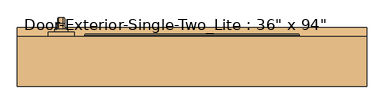
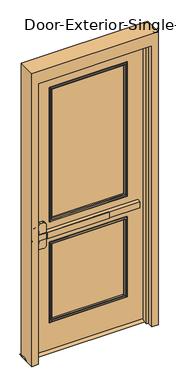
"""IFC4 building model written with IfcOpenShell, lengths in millimetres: door geometry."""

from ifc_helpers import new_model, si_unit, point, frame, frame_2d, origin, place, context, project, spatial, polyline, circle_curve, ellipse_curve, trimmed, segment, composite_curve, outline, extrude, faceted_brep, source, transform, mapped, element, save
from ifc_brep_helpers import plane_surface, cylinder_surface, revolved_surface, advanced_brep


def door_b6c2ee01(model_context):
    return source(origin(), model_context, "Body", "SolidModel", [
        extrude(outline(polyline([(38.1, 12.7), (82.55, 12.7), (107.95, 0.0), (12.7, 0.0), (38.1, 12.7)])), frame((-508.0, 0.0, 0.0), z_axis=(1.0, 0.0, 0.0), x_axis=(0.0, 1.0, 0.0)), (0.0, 0.0, 1.0), 1016.0),
        extrude(outline(polyline([(150.2833333, 0.0), (-349.25, 0.0), (-349.25, 6.35), (150.2833333, 6.35), (150.2833333, 0.0)])), frame((0.0, 0.0, 990.6), z_axis=(0.0, 0.0, 1.0), x_axis=(1.0, 0.0, 0.0)), (0.0, 0.0, 1.0), 50.8),
        advanced_brep(
        [(-412.75, 6.35, 1041.4), (-412.75, 6.35, 990.6), (-349.25, 6.35, 990.6), (400.05, 6.35, 990.6), (400.05, 6.35, 1041.4), (-349.25, 6.35, 1041.4), (400.05, 38.1, 1041.4), (400.05, 38.1, 990.6), (-349.25, 38.1, 990.6), (-349.25, 38.1, 927.1), (-368.3, 38.1, 908.05), (-393.7, 38.1, 908.05), (-412.75, 38.1, 927.1), (-412.75, 38.1, 1104.9), (-393.7, 38.1, 1123.95), (-368.3, 38.1, 1123.95), (-349.25, 38.1, 1104.9), (-349.25, 38.1, 1041.4), (-349.25, 9.5252467, 1041.4), (-412.75, 9.5252467, 1041.4), (-412.75, 14.5354269, 1104.9), (-412.75, 14.5354269, 927.1), (-412.75, 9.5252467, 990.6), (-349.25, 9.5252467, 990.6), (-349.25, 14.5354269, 927.1), (-349.25, 14.5354269, 1104.9), (-393.7, 16.038481, 1123.95), (-368.3, 16.038481, 1123.95), (-368.3, 16.038481, 908.05), (-393.7, 16.038481, 908.05)],
        [
            (0, 1),
            (1, 2),
            (2, 3),
            (3, 4),
            (4, 5),
            (5, 0),
            (6, 7),
            (7, 8),
            (8, 9),
            (9, 10, circle_curve(frame((-368.3, 38.1, 927.1), z_axis=(0.0, 1.0, 0.0), x_axis=(1.0, 0.0, 0.0)), 19.05)),
            (10, 11),
            (11, 12, circle_curve(frame((-393.7, 38.1, 927.1), z_axis=(0.0, 1.0, 0.0), x_axis=(1.0, 0.0, 0.0)), 19.05)),
            (12, 13),
            (13, 14, circle_curve(frame((-393.7, 38.1, 1104.9), z_axis=(0.0, 1.0, 0.0), x_axis=(1.0, 0.0, 0.0)), 19.05)),
            (14, 15),
            (15, 16, circle_curve(frame((-368.3, 38.1, 1104.9), z_axis=(0.0, 1.0, 0.0), x_axis=(1.0, 0.0, 0.0)), 19.05)),
            (16, 17),
            (17, 6),
            (4, 6),
            (17, 18),
            (18, 19),
            (19, 0),
            (19, 20),
            (20, 13),
            (12, 21),
            (21, 22),
            (22, 1),
            (7, 3),
            (22, 23),
            (23, 8),
            (23, 24),
            (24, 9),
            (16, 25),
            (25, 18),
            (14, 26),
            (26, 27),
            (27, 15),
            (10, 28),
            (28, 29),
            (29, 11),
            (24, 28, ellipse_curve(frame((-368.3, 14.5354269, 927.1), z_axis=(0.0, 0.9969018152893365, 0.07865602756830282), x_axis=(0.0, -0.07865602756830208, 0.9969018152893365)), 19.1092038, 19.05)),
            (27, 25, ellipse_curve(frame((-368.3, 14.5354269, 1104.9), z_axis=(0.0, 0.9969018152893376, -0.07865602756828934), x_axis=(0.0, -0.078656027568288, -0.9969018152893377)), 19.1092038, 19.05)),
            (20, 26, ellipse_curve(frame((-393.7, 14.5354269, 1104.9), z_axis=(0.0, 0.9969018152893376, -0.07865602756828934), x_axis=(0.0, -0.078656027568288, -0.9969018152893377)), 19.1092038, 19.05)),
            (29, 21, ellipse_curve(frame((-393.7, 14.5354269, 927.1), z_axis=(0.0, 0.9969018152893365, 0.07865602756830282), x_axis=(0.0, -0.07865602756830208, 0.9969018152893365)), 19.1092038, 19.05)),
        ],
        [
            plane_surface(frame((-412.75, 6.35, 1041.4), z_axis=(0.0, -1.0, 0.0), x_axis=(-1.0, 0.0, 0.0))),
            plane_surface(frame((-412.75, 38.1, 1041.4), z_axis=(0.0, 1.0, 0.0), x_axis=(1.0, 0.0, 0.0))),
            plane_surface(frame((400.05, 6.35, 1041.4), z_axis=(0.0, 0.0, 1.0), x_axis=(0.0, 1.0, 0.0))),
            plane_surface(frame((-412.75, 6.35, 1041.4), z_axis=(-1.0, 0.0, 0.0), x_axis=(0.0, 1.0, 0.0))),
            plane_surface(frame((-412.75, 6.35, 990.6), z_axis=(0.0, 0.0, -1.0), x_axis=(0.0, 1.0, 0.0))),
            plane_surface(frame((400.05, 6.35, 990.6), z_axis=(1.0, 0.0, 0.0), x_axis=(0.0, 1.0, 0.0))),
            plane_surface(frame((-349.25, 9.5252467, 927.1), z_axis=(1.0, 0.0, 0.0), x_axis=(0.0, 1.0, 0.0))),
            plane_surface(frame((-368.3, 9.5252467, 1123.95), z_axis=(0.0, 0.0, 1.0), x_axis=(0.0, 1.0, 0.0))),
            plane_surface(frame((-393.7, 9.5252467, 908.05), z_axis=(0.0, 0.0, -1.0), x_axis=(0.0, 1.0, 0.0))),
            cylinder_surface(frame((-368.3, 38.1, 927.1), z_axis=(0.0, -1.0, 0.0), x_axis=(1.0, 0.0, 0.0)), 19.05),
            cylinder_surface(frame((-368.3, 38.1, 1104.9), z_axis=(0.0, -1.0, 0.0), x_axis=(1.0, 0.0, 0.0)), 19.05),
            cylinder_surface(frame((-393.7, 38.1, 1104.9), z_axis=(0.0, -1.0, 0.0), x_axis=(1.0, 0.0, 0.0)), 19.05),
            cylinder_surface(frame((-393.7, 38.1, 927.1), z_axis=(0.0, -1.0, 0.0), x_axis=(1.0, 0.0, 0.0)), 19.05),
            plane_surface(frame((-349.25, 9.5252467, 1041.4), z_axis=(0.0, -0.9969018152893376, 0.07865602756828934), x_axis=(-1.0, 0.0, 0.0))),
            plane_surface(frame((-349.25, 16.038481, 908.05), z_axis=(0.0, -0.9969018152893365, -0.07865602756830282), x_axis=(-1.0, 0.0, 0.0))),
        ],
        [
            (0, [[1, 2, 3, 4, 5, 6]]),
            (1, [[7, 8, 9, 10, 11, 12, 13, 14, 15, 16, 17, 18]]),
            (2, [[19, -18, 20, 21, 22, -6, -5]]),
            (3, [[-1, -22, 23, 24, -13, 25, 26, 27]]),
            (4, [[28, -3, -2, -27, 29, 30, -8]]),
            (5, [[-4, -28, -7, -19]]),
            (6, [[-9, -30, 31, 32]]),
            (6, [[-17, 33, 34, -20]]),
            (7, [[-15, 35, 36, 37]]),
            (8, [[-11, 38, 39, 40]]),
            (9, [[-10, -32, 41, -38]]),
            (10, [[-16, -37, 42, -33]]),
            (11, [[-14, -24, 43, -35]]),
            (12, [[-12, -40, 44, -25]]),
            (13, [[-21, -34, -42, -36, -43, -23]]),
            (14, [[-26, -44, -39, -41, -31, -29]]),
        ],
    ),
        advanced_brep(
        [(-391.0, 95.25, 1017.190625), (-391.0, 95.25, 1014.809375), (-387.428125, 95.25, 1011.2375), (-374.5715406, 95.25, 1011.2375), (-371.0, 95.25, 1014.8090406), (-371.0, 95.25, 1017.190625), (-374.571875, 95.25, 1020.7625), (-387.428125, 95.25, 1020.7625), (-391.0, 95.25, 887.809375), (-387.428125, 95.25, 884.2375), (-374.571875, 95.25, 884.2375), (-371.0, 95.25, 887.809375), (-371.0, 95.25, 890.1909594), (-374.5715406, 95.25, 893.7625), (-387.428125, 95.25, 893.7625), (-391.0, 95.25, 890.190625), (-391.0, 120.65, 1017.190625), (-391.0, 134.540625, 1003.3), (-391.0, 134.540625, 901.7), (-391.0, 120.65, 887.809375), (-391.0, 120.65, 890.190625), (-391.0, 132.159375, 901.7), (-391.0, 132.159375, 1003.3), (-391.0, 120.65, 1014.809375), (-387.428125, 120.65, 1011.2375), (-374.5715406, 120.65, 1011.2375), (-371.0, 120.65, 1014.8090406), (-371.0, 132.1590406, 1003.3), (-371.0, 132.1590406, 901.7), (-371.0, 120.65, 890.1909594), (-371.0, 120.65, 887.809375), (-371.0, 134.540625, 901.7), (-371.0, 134.540625, 1003.3), (-371.0, 120.65, 1017.190625), (-374.571875, 120.65, 1020.7625), (-387.428125, 120.65, 1020.7625), (-387.428125, 128.5875, 1003.3), (-374.5715406, 128.5875, 1003.3), (-374.571875, 138.1125, 1003.3), (-387.428125, 138.1125, 1003.3), (-387.428125, 128.5875, 901.7), (-374.5715406, 128.5875, 901.7), (-374.571875, 138.1125, 901.7), (-387.428125, 138.1125, 901.7), (-387.428125, 120.65, 893.7625), (-374.5715406, 120.65, 893.7625), (-374.571875, 120.65, 884.2375), (-387.428125, 120.65, 884.2375)],
        [
            (0, 1),
            (1, 2, circle_curve(frame((-387.428125, 95.25, 1014.809375), z_axis=(0.0, -1.0, 0.0), x_axis=(0.0, 0.0, 1.0)), 3.571875)),
            (2, 3),
            (3, 4, circle_curve(frame((-374.5715406, 95.25, 1014.8090406), z_axis=(0.0, -1.0, 0.0), x_axis=(0.0, 0.0, 1.0)), 3.5715406)),
            (4, 5),
            (5, 6, circle_curve(frame((-374.571875, 95.25, 1017.190625), z_axis=(0.0, -1.0, 0.0), x_axis=(0.0, 0.0, 1.0)), 3.571875)),
            (6, 7),
            (7, 0, circle_curve(frame((-387.428125, 95.25, 1017.190625), z_axis=(0.0, -1.0, 0.0), x_axis=(0.0, 0.0, 1.0)), 3.571875)),
            (8, 9, circle_curve(frame((-387.428125, 95.25, 887.809375), z_axis=(0.0, -1.0, 0.0), x_axis=(0.0, 0.0, -1.0)), 3.571875)),
            (9, 10),
            (10, 11, circle_curve(frame((-374.571875, 95.25, 887.809375), z_axis=(0.0, -1.0, 0.0), x_axis=(0.0, 0.0, -1.0)), 3.571875)),
            (11, 12),
            (12, 13, circle_curve(frame((-374.5715406, 95.25, 890.1909594), z_axis=(0.0, -1.0, 0.0), x_axis=(0.0, 0.0, -1.0)), 3.5715406)),
            (13, 14),
            (14, 15, circle_curve(frame((-387.428125, 95.25, 890.190625), z_axis=(0.0, -1.0, 0.0), x_axis=(0.0, 0.0, -1.0)), 3.571875)),
            (15, 8),
            (0, 16),
            (16, 17, circle_curve(frame((-391.0, 120.65, 1003.3), z_axis=(-1.0, 0.0, 0.0), x_axis=(0.0, 0.0, 1.0)), 13.890625)),
            (17, 18),
            (18, 19, circle_curve(frame((-391.0, 120.65, 901.7), z_axis=(-1.0, 0.0, 0.0), x_axis=(0.0, 1.0, 0.0)), 13.890625)),
            (19, 8),
            (15, 20),
            (20, 21, circle_curve(frame((-391.0, 120.65, 901.7), z_axis=(1.0, 0.0, 0.0), x_axis=(0.0, 1.0, 0.0)), 11.509375)),
            (21, 22),
            (22, 23, circle_curve(frame((-391.0, 120.65, 1003.3), z_axis=(1.0, 0.0, 0.0), x_axis=(0.0, 0.0, 1.0)), 11.509375)),
            (23, 1),
            (23, 24, circle_curve(frame((-387.428125, 120.65, 1014.809375), z_axis=(0.0, -1.0, 0.0), x_axis=(0.0, 0.0, 1.0)), 3.571875)),
            (24, 2),
            (24, 25),
            (25, 3),
            (25, 26, circle_curve(frame((-374.5715406, 120.65, 1014.8090406), z_axis=(0.0, -1.0, 0.0), x_axis=(0.0, 0.0, 1.0)), 3.5715406)),
            (26, 4),
            (26, 27, circle_curve(frame((-371.0, 120.65, 1003.3), z_axis=(-1.0, 0.0, 0.0), x_axis=(0.0, 0.0, 1.0)), 11.5090406)),
            (27, 28),
            (28, 29, circle_curve(frame((-371.0, 120.65, 901.7), z_axis=(-1.0, 0.0, 0.0), x_axis=(0.0, 1.0, 0.0)), 11.5090406)),
            (29, 12),
            (11, 30),
            (30, 31, circle_curve(frame((-371.0, 120.65, 901.7), z_axis=(1.0, 0.0, 0.0), x_axis=(0.0, 1.0, 0.0)), 13.890625)),
            (31, 32),
            (32, 33, circle_curve(frame((-371.0, 120.65, 1003.3), z_axis=(1.0, 0.0, 0.0), x_axis=(0.0, 0.0, 1.0)), 13.890625)),
            (33, 5),
            (33, 34, circle_curve(frame((-374.571875, 120.65, 1017.190625), z_axis=(0.0, -1.0, 0.0), x_axis=(0.0, 0.0, 1.0)), 3.571875)),
            (34, 6),
            (34, 35),
            (35, 7),
            (35, 16, circle_curve(frame((-387.428125, 120.65, 1017.190625), z_axis=(0.0, -1.0, 0.0), x_axis=(0.0, 0.0, 1.0)), 3.571875)),
            (36, 24, circle_curve(frame((-387.428125, 120.65, 1003.3), z_axis=(1.0, 0.0, 0.0), x_axis=(0.0, 0.0, 1.0)), 7.9375)),
            (22, 36, circle_curve(frame((-387.428125, 132.159375, 1003.3), z_axis=(0.0, 0.0, 1.0), x_axis=(0.0, 1.0, 0.0)), 3.571875)),
            (37, 25, circle_curve(frame((-374.5715406, 120.65, 1003.3), z_axis=(1.0, 0.0, 0.0), x_axis=(0.0, 0.0, 1.0)), 7.9375)),
            (36, 37),
            (37, 27, circle_curve(frame((-374.5715406, 132.1590406, 1003.3), z_axis=(0.0, 0.0, 1.0), x_axis=(0.0, 1.0, 0.0)), 3.5715406)),
            (38, 34, circle_curve(frame((-374.571875, 120.65, 1003.3), z_axis=(1.0, 0.0, 0.0), x_axis=(0.0, 0.0, 1.0)), 17.4625)),
            (32, 38, circle_curve(frame((-374.571875, 134.540625, 1003.3), z_axis=(0.0, 0.0, 1.0), x_axis=(0.0, 1.0, 0.0)), 3.571875)),
            (39, 35, circle_curve(frame((-387.428125, 120.65, 1003.3), z_axis=(1.0, 0.0, 0.0), x_axis=(0.0, 0.0, 1.0)), 17.4625)),
            (38, 39),
            (39, 17, circle_curve(frame((-387.428125, 134.540625, 1003.3), z_axis=(0.0, 0.0, 1.0), x_axis=(0.0, 1.0, 0.0)), 3.571875)),
            (21, 40, circle_curve(frame((-387.428125, 132.159375, 901.7), z_axis=(0.0, 0.0, 1.0), x_axis=(0.0, 1.0, 0.0)), 3.571875)),
            (40, 36),
            (40, 41),
            (41, 37),
            (41, 28, circle_curve(frame((-374.5715406, 132.1590406, 901.7), z_axis=(0.0, 0.0, 1.0), x_axis=(0.0, 1.0, 0.0)), 3.5715406)),
            (31, 42, circle_curve(frame((-374.571875, 134.540625, 901.7), z_axis=(0.0, 0.0, 1.0), x_axis=(0.0, 1.0, 0.0)), 3.571875)),
            (42, 38),
            (42, 43),
            (43, 39),
            (43, 18, circle_curve(frame((-387.428125, 134.540625, 901.7), z_axis=(0.0, 0.0, 1.0), x_axis=(0.0, 1.0, 0.0)), 3.571875)),
            (44, 40, circle_curve(frame((-387.428125, 120.65, 901.7), z_axis=(1.0, 0.0, 0.0), x_axis=(0.0, 1.0, 0.0)), 7.9375)),
            (20, 44, circle_curve(frame((-387.428125, 120.65, 890.190625), z_axis=(0.0, 1.0, 0.0), x_axis=(0.0, 0.0, -1.0)), 3.571875)),
            (45, 41, circle_curve(frame((-374.5715406, 120.65, 901.7), z_axis=(1.0, 0.0, 0.0), x_axis=(0.0, 1.0, 0.0)), 7.9375)),
            (44, 45),
            (45, 29, circle_curve(frame((-374.5715406, 120.65, 890.1909594), z_axis=(0.0, 1.0, 0.0), x_axis=(0.0, 0.0, -1.0)), 3.5715406)),
            (46, 42, circle_curve(frame((-374.571875, 120.65, 901.7), z_axis=(1.0, 0.0, 0.0), x_axis=(0.0, 1.0, 0.0)), 17.4625)),
            (30, 46, circle_curve(frame((-374.571875, 120.65, 887.809375), z_axis=(0.0, 1.0, 0.0), x_axis=(0.0, 0.0, -1.0)), 3.571875)),
            (47, 43, circle_curve(frame((-387.428125, 120.65, 901.7), z_axis=(1.0, 0.0, 0.0), x_axis=(0.0, 1.0, 0.0)), 17.4625)),
            (46, 47),
            (47, 19, circle_curve(frame((-387.428125, 120.65, 887.809375), z_axis=(0.0, 1.0, 0.0), x_axis=(0.0, 0.0, -1.0)), 3.571875)),
            (14, 44),
            (13, 45),
            (10, 46),
            (9, 47),
        ],
        [
            plane_surface(frame((-381.0, 95.25, 1016.0), z_axis=(0.0, -1.0, 0.0), x_axis=(1.0, 0.0, 0.0))),
            plane_surface(frame((-381.0, 95.25, 889.0), z_axis=(0.0, -1.0, 0.0), x_axis=(1.0, 0.0, 0.0))),
            plane_surface(frame((-391.0, 95.25, 1017.190625), z_axis=(-1.0, 0.0, 0.0), x_axis=(0.0, 1.0, 0.0))),
            cylinder_surface(frame((-387.428125, 95.25, 1014.809375), z_axis=(0.0, -1.0, 0.0), x_axis=(0.0, 0.0, 1.0)), 3.571875),
            plane_surface(frame((-387.428125, 95.25, 1011.2375), z_axis=(0.0, 0.0, -1.0), x_axis=(0.0, 1.0, 0.0))),
            cylinder_surface(frame((-374.5715406, 95.25, 1014.8090406), z_axis=(0.0, -1.0, 0.0), x_axis=(0.0, 0.0, 1.0)), 3.5715406),
            plane_surface(frame((-371.0, 95.25, 1014.8090406), z_axis=(1.0, 0.0, 0.0), x_axis=(0.0, 1.0, 0.0))),
            cylinder_surface(frame((-374.571875, 95.25, 1017.190625), z_axis=(0.0, -1.0, 0.0), x_axis=(0.0, 0.0, 1.0)), 3.571875),
            plane_surface(frame((-374.571875, 95.25, 1020.7625), z_axis=(0.0, 0.0, 1.0), x_axis=(0.0, 1.0, 0.0))),
            cylinder_surface(frame((-387.428125, 95.25, 1017.190625), z_axis=(0.0, -1.0, 0.0), x_axis=(0.0, 0.0, 1.0)), 3.571875),
            revolved_surface(trimmed(ellipse_curve(frame((-387.428125, 120.65, 1014.809375), z_axis=(0.0, -1.0, 0.0), x_axis=(0.0, 0.0, 1.0)), 3.571875, 3.571875), [point((-391.0, 120.65, 1014.809375))], [point((-387.428125, 120.65, 1011.2375))], True, "CARTESIAN"), (-381.0, 120.65, 1003.3), (-1.0, 0.0, 0.0)),
            revolved_surface(polyline([(-387.428125, 120.65, 1011.2375), (-374.5715406, 120.65, 1011.2375)]), (-381.0, 120.65, 1003.3), (-1.0, 0.0, 0.0)),
            revolved_surface(trimmed(ellipse_curve(frame((-374.5715406, 120.65, 1014.8090406), z_axis=(0.0, -1.0, 0.0), x_axis=(0.0, 0.0, 1.0)), 3.5715406, 3.5715406), [point((-374.5715406, 120.65, 1011.2375))], [point((-371.0, 120.65, 1014.8090406))], True, "CARTESIAN"), (-381.0, 120.65, 1003.3), (-1.0, 0.0, 0.0)),
            revolved_surface(trimmed(ellipse_curve(frame((-374.571875, 120.65, 1017.190625), z_axis=(0.0, -1.0, 0.0), x_axis=(0.0, 0.0, 1.0)), 3.571875, 3.571875), [point((-371.0, 120.65, 1017.190625))], [point((-374.571875, 120.65, 1020.7625))], True, "CARTESIAN"), (-381.0, 120.65, 1003.3), (-1.0, 0.0, 0.0)),
            cylinder_surface(frame((-381.0, 120.65, 1003.3), z_axis=(-1.0, 0.0, 0.0), x_axis=(0.0, 0.0, 1.0)), 17.4625),
            revolved_surface(trimmed(ellipse_curve(frame((-387.428125, 120.65, 1017.190625), z_axis=(0.0, -1.0, 0.0), x_axis=(0.0, 0.0, 1.0)), 3.571875, 3.571875), [point((-387.428125, 120.65, 1020.7625))], [point((-391.0, 120.65, 1017.190625))], True, "CARTESIAN"), (-381.0, 120.65, 1003.3), (-1.0, 0.0, 0.0)),
            cylinder_surface(frame((-387.428125, 132.159375, 1003.3), z_axis=(0.0, 0.0, 1.0), x_axis=(0.0, 1.0, 0.0)), 3.571875),
            plane_surface(frame((-387.428125, 128.5875, 1003.3), z_axis=(0.0, -1.0, 0.0), x_axis=(0.0, 0.0, -1.0))),
            cylinder_surface(frame((-374.5715406, 132.1590406, 1003.3), z_axis=(0.0, 0.0, 1.0), x_axis=(0.0, 1.0, 0.0)), 3.5715406),
            cylinder_surface(frame((-374.571875, 134.540625, 1003.3), z_axis=(0.0, 0.0, 1.0), x_axis=(0.0, 1.0, 0.0)), 3.571875),
            plane_surface(frame((-374.571875, 138.1125, 1003.3), z_axis=(0.0, 1.0, 0.0), x_axis=(0.0, 0.0, -1.0))),
            cylinder_surface(frame((-387.428125, 134.540625, 1003.3), z_axis=(0.0, 0.0, 1.0), x_axis=(0.0, 1.0, 0.0)), 3.571875),
            revolved_surface(trimmed(ellipse_curve(frame((-387.428125, 132.159375, 901.7), z_axis=(0.0, 0.0, 1.0), x_axis=(0.0, 1.0, 0.0)), 3.571875, 3.571875), [point((-391.0, 132.159375, 901.7))], [point((-387.428125, 128.5875, 901.7))], True, "CARTESIAN"), (-381.0, 120.65, 901.7), (-1.0, 0.0, 0.0)),
            revolved_surface(polyline([(-387.428125, 128.5875, 901.7), (-374.5715406, 128.5875, 901.7)]), (-381.0, 120.65, 901.7), (-1.0, 0.0, 0.0)),
            revolved_surface(trimmed(ellipse_curve(frame((-374.5715406, 132.1590406, 901.7), z_axis=(0.0, 0.0, 1.0), x_axis=(0.0, 1.0, 0.0)), 3.5715406, 3.5715406), [point((-374.5715406, 128.5875, 901.7))], [point((-371.0, 132.1590406, 901.7))], True, "CARTESIAN"), (-381.0, 120.65, 901.7), (-1.0, 0.0, 0.0)),
            revolved_surface(trimmed(ellipse_curve(frame((-374.571875, 134.540625, 901.7), z_axis=(0.0, 0.0, 1.0), x_axis=(0.0, 1.0, 0.0)), 3.571875, 3.571875), [point((-371.0, 134.540625, 901.7))], [point((-374.571875, 138.1125, 901.7))], True, "CARTESIAN"), (-381.0, 120.65, 901.7), (-1.0, 0.0, 0.0)),
            cylinder_surface(frame((-381.0, 120.65, 901.7), z_axis=(-1.0, 0.0, 0.0), x_axis=(0.0, 1.0, 0.0)), 17.4625),
            revolved_surface(trimmed(ellipse_curve(frame((-387.428125, 134.540625, 901.7), z_axis=(0.0, 0.0, 1.0), x_axis=(0.0, 1.0, 0.0)), 3.571875, 3.571875), [point((-387.428125, 138.1125, 901.7))], [point((-391.0, 134.540625, 901.7))], True, "CARTESIAN"), (-381.0, 120.65, 901.7), (-1.0, 0.0, 0.0)),
            cylinder_surface(frame((-387.428125, 120.65, 890.190625), z_axis=(0.0, 1.0, 0.0), x_axis=(0.0, 0.0, -1.0)), 3.571875),
            plane_surface(frame((-387.428125, 120.65, 893.7625), z_axis=(0.0, 0.0, 1.0), x_axis=(0.0, -1.0, 0.0))),
            cylinder_surface(frame((-374.5715406, 120.65, 890.1909594), z_axis=(0.0, 1.0, 0.0), x_axis=(0.0, 0.0, -1.0)), 3.5715406),
            cylinder_surface(frame((-374.571875, 120.65, 887.809375), z_axis=(0.0, 1.0, 0.0), x_axis=(0.0, 0.0, -1.0)), 3.571875),
            plane_surface(frame((-374.571875, 120.65, 884.2375), z_axis=(0.0, 0.0, -1.0), x_axis=(0.0, -1.0, 0.0))),
            cylinder_surface(frame((-387.428125, 120.65, 887.809375), z_axis=(0.0, 1.0, 0.0), x_axis=(0.0, 0.0, -1.0)), 3.571875),
        ],
        [
            (0, [[1, 2, 3, 4, 5, 6, 7, 8]]),
            (1, [[9, 10, 11, 12, 13, 14, 15, 16]]),
            (2, [[-1, 17, 18, 19, 20, 21, -16, 22, 23, 24, 25, 26]]),
            (3, [[-2, -26, 27, 28]]),
            (4, [[-3, -28, 29, 30]]),
            (5, [[-4, -30, 31, 32]]),
            (6, [[-5, -32, 33, 34, 35, 36, -12, 37, 38, 39, 40, 41]]),
            (7, [[-6, -41, 42, 43]]),
            (8, [[-7, -43, 44, 45]]),
            (9, [[-8, -45, 46, -17]]),
            (10, [[47, -27, -25, 48]]),
            (11, [[49, -29, -47, 50]]),
            (12, [[-33, -31, -49, 51]]),
            (13, [[52, -42, -40, 53]]),
            (14, [[54, -44, -52, 55]]),
            (15, [[-18, -46, -54, 56]]),
            (16, [[-48, -24, 57, 58]]),
            (17, [[-50, -58, 59, 60]]),
            (18, [[-51, -60, 61, -34]]),
            (19, [[-53, -39, 62, 63]]),
            (20, [[-55, -63, 64, 65]]),
            (21, [[-56, -65, 66, -19]]),
            (22, [[67, -57, -23, 68]]),
            (23, [[69, -59, -67, 70]]),
            (24, [[-35, -61, -69, 71]]),
            (25, [[72, -62, -38, 73]]),
            (26, [[74, -64, -72, 75]]),
            (27, [[-20, -66, -74, 76]]),
            (28, [[-68, -22, -15, 77]]),
            (29, [[-70, -77, -14, 78]]),
            (30, [[-71, -78, -13, -36]]),
            (31, [[-73, -37, -11, 79]]),
            (32, [[-75, -79, -10, 80]]),
            (33, [[-76, -80, -9, -21]]),
        ],
    ),
        extrude(outline(composite_curve([segment(trimmed(circle_curve(frame_2d((1117.6, -381.0)), 19.0), [point((1117.6, -400.0))], [point((1117.6, -362.0))], False, "CARTESIAN"), True, "CONTINUOUS"), segment(trimmed(circle_curve(frame_2d((1117.6, -381.0)), 19.0), [point((1117.6, -362.0))], [point((1117.6, -400.0))], False, "CARTESIAN"), True, "CONTINUOUS")], self_intersect=False)), frame((0.0, 95.25, 0.0), z_axis=(0.0, 1.0, 0.0), x_axis=(0.0, 0.0, 1.0)), (0.0, 0.0, 1.0), 8.73125),
        extrude(outline(composite_curve([segment(trimmed(circle_curve(frame_2d((1113.0338574, -381.0)), 89.3016225), [point((1193.8, -342.9))], [point((1193.8, -419.1))], False, "CARTESIAN"), True, "CONTINUOUS"), segment(polyline([(1193.8, -419.1), (838.2, -419.1)]), True, "CONTINUOUS"), segment(trimmed(circle_curve(frame_2d((918.9661426, -381.0)), 89.3016225), [point((838.2, -419.1))], [point((838.2, -342.9))], False, "CARTESIAN"), True, "CONTINUOUS"), segment(polyline([(838.2, -342.9), (1193.8, -342.9)]), True, "CONTINUOUS")], self_intersect=False)), frame((0.0, 82.55, 0.0), z_axis=(0.0, 1.0, 0.0), x_axis=(0.0, 0.0, 1.0)), (0.0, 0.0, 1.0), 12.7),
        faceted_brep([(457.2, 33.3375, 0.0), (457.2, 82.55, 0.0), (508.0, 82.55, 0.0), (508.0, -63.5, 0.0), (457.2, -63.5, 0.0), (457.2, -14.2875, 0.0), (441.325, -14.2875, 0.0), (441.325, 33.3375, 0.0), (457.2, 33.3375, 2387.6), (457.2, 82.55, 2387.6), (-457.2, 82.55, 2387.6), (-457.2, 82.55, 0.0), (-508.0, 82.55, 0.0), (-508.0, 82.55, 2489.2), (508.0, 82.55, 2489.2), (508.0, -63.5, 2489.2), (-508.0, -63.5, 2489.2), (-508.0, -63.5, 0.0), (-457.2, -63.5, 0.0), (-457.2, -63.5, 2387.6), (457.2, -63.5, 2387.6), (457.2, -14.2875, 2387.6), (-457.2, -14.2875, 2387.6), (-457.2, -14.2875, 0.0), (-441.325, -14.2875, 0.0), (-441.325, -14.2875, 2371.725), (441.325, -14.2875, 2371.725), (441.325, 33.3375, 2371.725), (-441.325, 33.3375, 2371.725), (-441.325, 33.3375, 0.0), (-457.2, 33.3375, 0.0), (-457.2, 33.3375, 2387.6)], [[[0, 1, 2, 3, 4, 5, 6, 7]], [[1, 0, 8, 9]], [[2, 1, 9, 10, 11, 12, 13, 14]], [[3, 2, 14, 15]], [[4, 3, 15, 16, 17, 18, 19, 20]], [[5, 4, 20, 21]], [[6, 5, 21, 22, 23, 24, 25, 26]], [[7, 6, 26, 27]], [[0, 7, 27, 28, 29, 30, 31, 8]], [[9, 8, 31, 10]], [[20, 19, 22, 21]], [[26, 25, 28, 27]], [[12, 11, 30, 29, 24, 23, 18, 17]], [[11, 10, 31, 30]], [[13, 12, 17, 16]], [[19, 18, 23, 22]], [[25, 24, 29, 28]], [[15, 14, 13, 16]]]),
        extrude(outline(polyline([(2387.6, -457.2), (12.7, -457.2), (12.7, 457.2), (2387.6, 457.2), (2387.6, -457.2)]), holes=[polyline([(2235.2, -304.8), (2235.2, 304.8), (1111.25, 304.8), (1111.25, -304.8), (2235.2, -304.8)]), polyline([(920.75, -304.8), (920.75, 304.8), (254.0, 304.8), (254.0, -304.8), (920.75, -304.8)])]), frame((0.0, 38.1, 0.0), z_axis=(0.0, 1.0, 0.0), x_axis=(0.0, 0.0, 1.0)), (0.0, 0.0, 1.0), 44.45),
        extrude(outline(polyline([(304.8, 50.8), (-304.8, 50.8), (-304.8, 69.85), (304.8, 69.85), (304.8, 50.8)])), frame((0.0, 0.0, 1111.25), z_axis=(0.0, 0.0, 1.0), x_axis=(1.0, 0.0, 0.0)), (0.0, 0.0, 1.0), 1123.95),
        extrude(outline(polyline([(304.8, 50.8), (-304.8, 50.8), (-304.8, 69.85), (304.8, 69.85), (304.8, 50.8)])), frame((0.0, 0.0, 254.0), z_axis=(0.0, 0.0, 1.0), x_axis=(1.0, 0.0, 0.0)), (0.0, 0.0, 1.0), 666.75),
        advanced_brep(
        [(304.8, 50.8, 920.75), (304.8, 38.1, 920.75), (304.8, 38.1, 254.0), (304.8, 50.8, 254.0), (292.8, 37.1, 908.75), (292.8, 50.8, 908.75), (292.8, 50.8, 266.0), (292.8, 37.1, 266.0), (297.8, 32.1, 913.75), (297.8, 32.1, 261.0), (312.8, 34.1, 928.75), (310.8, 32.1, 926.75), (310.8, 32.1, 248.0), (312.8, 34.1, 246.0), (312.8, 38.1, 928.75), (312.8, 38.1, 246.0), (-304.8, 38.1, 254.0), (-304.8, 50.8, 254.0), (-292.8, 50.8, 266.0), (-292.8, 37.1, 266.0), (-297.8, 32.1, 261.0), (-310.8, 32.1, 248.0), (-312.8, 34.1, 246.0), (-312.8, 38.1, 246.0), (-304.8, 38.1, 920.75), (-304.8, 50.8, 920.75), (-292.8, 50.8, 908.75), (-292.8, 37.1, 908.75), (-297.8, 32.1, 913.75), (-310.8, 32.1, 926.75), (-312.8, 34.1, 928.75), (-312.8, 38.1, 928.75)],
        [
            (0, 1),
            (1, 2),
            (2, 3),
            (3, 0),
            (4, 5),
            (5, 6),
            (6, 7),
            (7, 4),
            (8, 4, ellipse_curve(frame((297.8, 37.1, 913.75), z_axis=(0.7071067811865475, 0.0, -0.7071067811865475), x_axis=(0.7071067811865474, 0.0, 0.7071067811865476)), 7.0710678, 5.0)),
            (7, 9, ellipse_curve(frame((297.8, 37.1, 261.0), z_axis=(0.7071067811865475, 0.0, 0.7071067811865475), x_axis=(-0.7071067811865474, 0.0, 0.7071067811865476)), 7.0710678, 5.0)),
            (9, 8),
            (10, 11, ellipse_curve(frame((310.8, 34.1, 926.75), z_axis=(0.7071067811865475, 0.0, -0.7071067811865475), x_axis=(0.7071067811865474, 0.0, 0.7071067811865476)), 2.8284271, 2.0)),
            (11, 12),
            (12, 13, ellipse_curve(frame((310.8, 34.1, 248.0), z_axis=(0.7071067811865475, 0.0, 0.7071067811865475), x_axis=(-0.7071067811865474, 0.0, 0.7071067811865476)), 2.8284271, 2.0)),
            (13, 10),
            (14, 10),
            (13, 15),
            (15, 14),
            (2, 16),
            (16, 17),
            (17, 3),
            (6, 18),
            (18, 19),
            (19, 7),
            (19, 20, ellipse_curve(frame((-297.8, 37.1, 261.0), z_axis=(0.7071067811865475, 0.0, -0.7071067811865475), x_axis=(0.7071067811865476, 0.0, 0.7071067811865474)), 7.0710678, 5.0)),
            (20, 9),
            (12, 21),
            (21, 22, ellipse_curve(frame((-310.8, 34.1, 248.0), z_axis=(0.7071067811865475, 0.0, -0.7071067811865475), x_axis=(0.7071067811865476, 0.0, 0.7071067811865474)), 2.8284271, 2.0)),
            (22, 13),
            (22, 23),
            (23, 15),
            (16, 24),
            (24, 25),
            (25, 17),
            (18, 26),
            (26, 27),
            (27, 19),
            (27, 28, ellipse_curve(frame((-297.8, 37.1, 913.75), z_axis=(-0.7071067811865475, 0.0, -0.7071067811865475), x_axis=(0.7071067811865474, 0.0, -0.7071067811865476)), 7.0710678, 5.0)),
            (28, 20),
            (21, 29),
            (29, 30, ellipse_curve(frame((-310.8, 34.1, 926.75), z_axis=(-0.7071067811865475, 0.0, -0.7071067811865475), x_axis=(0.7071067811865474, 0.0, -0.7071067811865476)), 2.8284271, 2.0)),
            (30, 22),
            (30, 31),
            (31, 23),
            (31, 14),
            (1, 24),
            (0, 25),
            (5, 26),
            (4, 27),
            (8, 28),
            (11, 29),
            (10, 30),
        ],
        [
            plane_surface(frame((304.8, 38.1, 920.75), z_axis=(1.0, 0.0, 0.0), x_axis=(0.0, 0.0, -1.0))),
            plane_surface(frame((292.8, 50.8, 908.75), z_axis=(-1.0, 0.0, 0.0), x_axis=(0.0, 0.0, -1.0))),
            cylinder_surface(frame((297.8, 37.1, 920.75), z_axis=(0.0, 0.0, 1.0), x_axis=(1.0, 0.0, 0.0)), 5.0),
            cylinder_surface(frame((310.8, 34.1, 920.75), z_axis=(0.0, 0.0, 1.0), x_axis=(1.0, 0.0, 0.0)), 2.0),
            plane_surface(frame((312.8, 34.1, 928.75), z_axis=(1.0, 0.0, 0.0), x_axis=(0.0, 0.0, -1.0))),
            plane_surface(frame((304.8, 38.1, 254.0), z_axis=(0.0, 0.0, -1.0), x_axis=(-1.0, 0.0, 0.0))),
            plane_surface(frame((292.8, 50.8, 266.0), z_axis=(0.0, 0.0, 1.0), x_axis=(-1.0, 0.0, 0.0))),
            cylinder_surface(frame((304.8, 37.1, 261.0), z_axis=(1.0, 0.0, 0.0), x_axis=(0.0, 0.0, -1.0)), 5.0),
            cylinder_surface(frame((304.8, 34.1, 248.0), z_axis=(1.0, 0.0, 0.0), x_axis=(0.0, 0.0, -1.0)), 2.0),
            plane_surface(frame((312.8, 34.1, 246.0), z_axis=(0.0, 0.0, -1.0), x_axis=(-1.0, 0.0, 0.0))),
            plane_surface(frame((-304.8, 38.1, 254.0), z_axis=(-1.0, 0.0, 0.0), x_axis=(0.0, 0.0, 1.0))),
            plane_surface(frame((-292.8, 50.8, 266.0), z_axis=(1.0, 0.0, 0.0), x_axis=(0.0, 0.0, 1.0))),
            cylinder_surface(frame((-297.8, 37.1, 254.0), z_axis=(0.0, 0.0, -1.0), x_axis=(-1.0, 0.0, 0.0)), 5.0),
            cylinder_surface(frame((-310.8, 34.1, 254.0), z_axis=(0.0, 0.0, -1.0), x_axis=(-1.0, 0.0, 0.0)), 2.0),
            plane_surface(frame((-312.8, 34.1, 246.0), z_axis=(-1.0, 0.0, 0.0), x_axis=(0.0, 0.0, 1.0))),
            plane_surface(frame((-312.8, 38.1, 928.75), z_axis=(0.0, 1.0, 0.0), x_axis=(1.0, 0.0, 0.0))),
            plane_surface(frame((-304.8, 38.1, 920.75), z_axis=(0.0, 0.0, 1.0), x_axis=(1.0, 0.0, 0.0))),
            plane_surface(frame((-304.8, 50.8, 920.75), z_axis=(0.0, 1.0, 0.0), x_axis=(1.0, 0.0, 0.0))),
            plane_surface(frame((-292.8, 50.8, 908.75), z_axis=(0.0, 0.0, -1.0), x_axis=(1.0, 0.0, 0.0))),
            cylinder_surface(frame((-304.8, 37.1, 913.75), z_axis=(-1.0, 0.0, 0.0), x_axis=(0.0, 0.0, 1.0)), 5.0),
            plane_surface(frame((-297.8, 32.1, 913.75), z_axis=(0.0, -1.0, 0.0), x_axis=(1.0, 0.0, 0.0))),
            cylinder_surface(frame((-304.8, 34.1, 926.75), z_axis=(-1.0, 0.0, 0.0), x_axis=(0.0, 0.0, 1.0)), 2.0),
            plane_surface(frame((-312.8, 34.1, 928.75), z_axis=(0.0, 0.0, 1.0), x_axis=(1.0, 0.0, 0.0))),
        ],
        [
            (0, [[1, 2, 3, 4]]),
            (1, [[5, 6, 7, 8]]),
            (2, [[9, -8, 10, 11]]),
            (3, [[12, 13, 14, 15]]),
            (4, [[16, -15, 17, 18]]),
            (5, [[-3, 19, 20, 21]]),
            (6, [[-7, 22, 23, 24]]),
            (7, [[-10, -24, 25, 26]]),
            (8, [[-14, 27, 28, 29]]),
            (9, [[-17, -29, 30, 31]]),
            (10, [[-20, 32, 33, 34]]),
            (11, [[-23, 35, 36, 37]]),
            (12, [[-25, -37, 38, 39]]),
            (13, [[-28, 40, 41, 42]]),
            (14, [[-30, -42, 43, 44]]),
            (15, [[-31, -44, 45, -18], [46, -32, -19, -2]]),
            (16, [[-33, -46, -1, 47]]),
            (17, [[-21, -34, -47, -4], [48, -35, -22, -6]]),
            (18, [[-36, -48, -5, 49]]),
            (19, [[-38, -49, -9, 50]]),
            (20, [[51, -40, -27, -13], [-26, -39, -50, -11]]),
            (21, [[-41, -51, -12, 52]]),
            (22, [[-43, -52, -16, -45]]),
        ],
    ),
        advanced_brep(
        [(-304.8, 69.85, 920.75), (-304.8, 82.55, 920.75), (-304.8, 82.55, 254.0), (-304.8, 69.85, 254.0), (-292.8, 83.55, 908.75), (-292.8, 69.85, 908.75), (-292.8, 69.85, 266.0), (-292.8, 83.55, 266.0), (-297.8, 88.55, 913.75), (-297.8, 88.55, 261.0), (-312.8, 86.55, 928.75), (-310.8, 88.55, 926.75), (-310.8, 88.55, 248.0), (-312.8, 86.55, 246.0), (-312.8, 82.55, 928.75), (-312.8, 82.55, 246.0), (304.8, 82.55, 254.0), (304.8, 69.85, 254.0), (292.8, 69.85, 266.0), (292.8, 83.55, 266.0), (297.8, 88.55, 261.0), (310.8, 88.55, 248.0), (312.8, 86.55, 246.0), (312.8, 82.55, 246.0), (304.8, 82.55, 920.75), (304.8, 69.85, 920.75), (292.8, 69.85, 908.75), (292.8, 83.55, 908.75), (297.8, 88.55, 913.75), (310.8, 88.55, 926.75), (312.8, 86.55, 928.75), (312.8, 82.55, 928.75)],
        [
            (0, 1),
            (1, 2),
            (2, 3),
            (3, 0),
            (4, 5),
            (5, 6),
            (6, 7),
            (7, 4),
            (8, 4, ellipse_curve(frame((-297.8, 83.55, 913.75), z_axis=(-0.7071067811865475, 0.0, -0.7071067811865475), x_axis=(-0.7071067811865474, 0.0, 0.7071067811865476)), 7.0710678, 5.0)),
            (7, 9, ellipse_curve(frame((-297.8, 83.55, 261.0), z_axis=(-0.7071067811865475, 0.0, 0.7071067811865475), x_axis=(0.7071067811865474, 0.0, 0.7071067811865476)), 7.0710678, 5.0)),
            (9, 8),
            (10, 11, ellipse_curve(frame((-310.8, 86.55, 926.75), z_axis=(-0.7071067811865475, 0.0, -0.7071067811865475), x_axis=(-0.7071067811865474, 0.0, 0.7071067811865476)), 2.8284271, 2.0)),
            (11, 12),
            (12, 13, ellipse_curve(frame((-310.8, 86.55, 248.0), z_axis=(-0.7071067811865475, 0.0, 0.7071067811865475), x_axis=(0.7071067811865474, 0.0, 0.7071067811865476)), 2.8284271, 2.0)),
            (13, 10),
            (14, 10),
            (13, 15),
            (15, 14),
            (2, 16),
            (16, 17),
            (17, 3),
            (6, 18),
            (18, 19),
            (19, 7),
            (19, 20, ellipse_curve(frame((297.8, 83.55, 261.0), z_axis=(-0.7071067811865475, 0.0, -0.7071067811865475), x_axis=(-0.7071067811865476, 0.0, 0.7071067811865474)), 7.0710678, 5.0)),
            (20, 9),
            (12, 21),
            (21, 22, ellipse_curve(frame((310.8, 86.55, 248.0), z_axis=(-0.7071067811865475, 0.0, -0.7071067811865475), x_axis=(-0.7071067811865476, 0.0, 0.7071067811865474)), 2.8284271, 2.0)),
            (22, 13),
            (22, 23),
            (23, 15),
            (16, 24),
            (24, 25),
            (25, 17),
            (18, 26),
            (26, 27),
            (27, 19),
            (27, 28, ellipse_curve(frame((297.8, 83.55, 913.75), z_axis=(0.7071067811865475, 0.0, -0.7071067811865475), x_axis=(-0.7071067811865474, 0.0, -0.7071067811865476)), 7.0710678, 5.0)),
            (28, 20),
            (21, 29),
            (29, 30, ellipse_curve(frame((310.8, 86.55, 926.75), z_axis=(0.7071067811865475, 0.0, -0.7071067811865475), x_axis=(-0.7071067811865474, 0.0, -0.7071067811865476)), 2.8284271, 2.0)),
            (30, 22),
            (30, 31),
            (31, 23),
            (31, 14),
            (1, 24),
            (0, 25),
            (5, 26),
            (4, 27),
            (8, 28),
            (11, 29),
            (10, 30),
        ],
        [
            plane_surface(frame((-304.8, 82.55, 920.75), z_axis=(-1.0, 0.0, 0.0), x_axis=(0.0, 0.0, -1.0))),
            plane_surface(frame((-292.8, 69.85, 908.75), z_axis=(1.0, 0.0, 0.0), x_axis=(0.0, 0.0, -1.0))),
            cylinder_surface(frame((-297.8, 83.55, 920.75), z_axis=(0.0, 0.0, 1.0), x_axis=(-1.0, 0.0, 0.0)), 5.0),
            cylinder_surface(frame((-310.8, 86.55, 920.75), z_axis=(0.0, 0.0, 1.0), x_axis=(-1.0, 0.0, 0.0)), 2.0),
            plane_surface(frame((-312.8, 86.55, 928.75), z_axis=(-1.0, 0.0, 0.0), x_axis=(0.0, 0.0, -1.0))),
            plane_surface(frame((-304.8, 82.55, 254.0), z_axis=(0.0, 0.0, -1.0), x_axis=(1.0, 0.0, 0.0))),
            plane_surface(frame((-292.8, 69.85, 266.0), z_axis=(0.0, 0.0, 1.0), x_axis=(1.0, 0.0, 0.0))),
            cylinder_surface(frame((-304.8, 83.55, 261.0), z_axis=(-1.0, 0.0, 0.0), x_axis=(0.0, 0.0, -1.0)), 5.0),
            cylinder_surface(frame((-304.8, 86.55, 248.0), z_axis=(-1.0, 0.0, 0.0), x_axis=(0.0, 0.0, -1.0)), 2.0),
            plane_surface(frame((-312.8, 86.55, 246.0), z_axis=(0.0, 0.0, -1.0), x_axis=(1.0, 0.0, 0.0))),
            plane_surface(frame((304.8, 82.55, 254.0), z_axis=(1.0, 0.0, 0.0), x_axis=(0.0, 0.0, 1.0))),
            plane_surface(frame((292.8, 69.85, 266.0), z_axis=(-1.0, 0.0, 0.0), x_axis=(0.0, 0.0, 1.0))),
            cylinder_surface(frame((297.8, 83.55, 254.0), z_axis=(0.0, 0.0, -1.0), x_axis=(1.0, 0.0, 0.0)), 5.0),
            cylinder_surface(frame((310.8, 86.55, 254.0), z_axis=(0.0, 0.0, -1.0), x_axis=(1.0, 0.0, 0.0)), 2.0),
            plane_surface(frame((312.8, 86.55, 246.0), z_axis=(1.0, 0.0, 0.0), x_axis=(0.0, 0.0, 1.0))),
            plane_surface(frame((312.8, 82.55, 928.75), z_axis=(0.0, -1.0, 0.0), x_axis=(-1.0, 0.0, 0.0))),
            plane_surface(frame((304.8, 82.55, 920.75), z_axis=(0.0, 0.0, 1.0), x_axis=(-1.0, 0.0, 0.0))),
            plane_surface(frame((304.8, 69.85, 920.75), z_axis=(0.0, -1.0, 0.0), x_axis=(-1.0, 0.0, 0.0))),
            plane_surface(frame((292.8, 69.85, 908.75), z_axis=(0.0, 0.0, -1.0), x_axis=(-1.0, 0.0, 0.0))),
            cylinder_surface(frame((304.8, 83.55, 913.75), z_axis=(1.0, 0.0, 0.0), x_axis=(0.0, 0.0, 1.0)), 5.0),
            plane_surface(frame((297.8, 88.55, 913.75), z_axis=(0.0, 1.0, 0.0), x_axis=(-1.0, 0.0, 0.0))),
            cylinder_surface(frame((304.8, 86.55, 926.75), z_axis=(1.0, 0.0, 0.0), x_axis=(0.0, 0.0, 1.0)), 2.0),
            plane_surface(frame((312.8, 86.55, 928.75), z_axis=(0.0, 0.0, 1.0), x_axis=(-1.0, 0.0, 0.0))),
        ],
        [
            (0, [[1, 2, 3, 4]]),
            (1, [[5, 6, 7, 8]]),
            (2, [[9, -8, 10, 11]]),
            (3, [[12, 13, 14, 15]]),
            (4, [[16, -15, 17, 18]]),
            (5, [[-3, 19, 20, 21]]),
            (6, [[-7, 22, 23, 24]]),
            (7, [[-10, -24, 25, 26]]),
            (8, [[-14, 27, 28, 29]]),
            (9, [[-17, -29, 30, 31]]),
            (10, [[-20, 32, 33, 34]]),
            (11, [[-23, 35, 36, 37]]),
            (12, [[-25, -37, 38, 39]]),
            (13, [[-28, 40, 41, 42]]),
            (14, [[-30, -42, 43, 44]]),
            (15, [[-31, -44, 45, -18], [46, -32, -19, -2]]),
            (16, [[-33, -46, -1, 47]]),
            (17, [[-21, -34, -47, -4], [48, -35, -22, -6]]),
            (18, [[-36, -48, -5, 49]]),
            (19, [[-38, -49, -9, 50]]),
            (20, [[51, -40, -27, -13], [-26, -39, -50, -11]]),
            (21, [[-41, -51, -12, 52]]),
            (22, [[-43, -52, -16, -45]]),
        ],
    ),
        advanced_brep(
        [(-304.8, 50.8, 1111.25), (-304.8, 38.1, 1111.25), (-304.8, 38.1, 2235.2), (-304.8, 50.8, 2235.2), (-292.8, 37.1, 1123.25), (-292.8, 50.8, 1123.25), (-292.8, 50.8, 2223.2), (-292.8, 37.1, 2223.2), (-297.8, 32.1, 1118.25), (-297.8, 32.1, 2228.2), (-312.8, 34.1, 1103.25), (-310.8, 32.1, 1105.25), (-310.8, 32.1, 2241.2), (-312.8, 34.1, 2243.2), (-312.8, 38.1, 1103.25), (-312.8, 38.1, 2243.2), (304.8, 38.1, 2235.2), (304.8, 50.8, 2235.2), (292.8, 50.8, 2223.2), (292.8, 37.1, 2223.2), (297.8, 32.1, 2228.2), (310.8, 32.1, 2241.2), (312.8, 34.1, 2243.2), (312.8, 38.1, 2243.2), (304.8, 38.1, 1111.25), (304.8, 50.8, 1111.25), (292.8, 50.8, 1123.25), (292.8, 37.1, 1123.25), (297.8, 32.1, 1118.25), (310.8, 32.1, 1105.25), (312.8, 34.1, 1103.25), (312.8, 38.1, 1103.25)],
        [
            (0, 1),
            (1, 2),
            (2, 3),
            (3, 0),
            (4, 5),
            (5, 6),
            (6, 7),
            (7, 4),
            (8, 4, ellipse_curve(frame((-297.8, 37.1, 1118.25), z_axis=(-0.7071067811865475, 0.0, 0.7071067811865475), x_axis=(-0.7071067811865474, 0.0, -0.7071067811865476)), 7.0710678, 5.0)),
            (7, 9, ellipse_curve(frame((-297.8, 37.1, 2228.2), z_axis=(-0.7071067811865475, 0.0, -0.7071067811865475), x_axis=(0.7071067811865474, 0.0, -0.7071067811865476)), 7.0710678, 5.0)),
            (9, 8),
            (10, 11, ellipse_curve(frame((-310.8, 34.1, 1105.25), z_axis=(-0.7071067811865475, 0.0, 0.7071067811865475), x_axis=(-0.7071067811865474, 0.0, -0.7071067811865476)), 2.8284271, 2.0)),
            (11, 12),
            (12, 13, ellipse_curve(frame((-310.8, 34.1, 2241.2), z_axis=(-0.7071067811865475, 0.0, -0.7071067811865475), x_axis=(0.7071067811865474, 0.0, -0.7071067811865476)), 2.8284271, 2.0)),
            (13, 10),
            (14, 10),
            (13, 15),
            (15, 14),
            (2, 16),
            (16, 17),
            (17, 3),
            (6, 18),
            (18, 19),
            (19, 7),
            (19, 20, ellipse_curve(frame((297.8, 37.1, 2228.2), z_axis=(-0.7071067811865475, 0.0, 0.7071067811865475), x_axis=(-0.7071067811865476, 0.0, -0.7071067811865474)), 7.0710678, 5.0)),
            (20, 9),
            (12, 21),
            (21, 22, ellipse_curve(frame((310.8, 34.1, 2241.2), z_axis=(-0.7071067811865475, 0.0, 0.7071067811865475), x_axis=(-0.7071067811865476, 0.0, -0.7071067811865474)), 2.8284271, 2.0)),
            (22, 13),
            (22, 23),
            (23, 15),
            (16, 24),
            (24, 25),
            (25, 17),
            (18, 26),
            (26, 27),
            (27, 19),
            (27, 28, ellipse_curve(frame((297.8, 37.1, 1118.25), z_axis=(0.7071067811865475, 0.0, 0.7071067811865475), x_axis=(-0.7071067811865474, 0.0, 0.7071067811865476)), 7.0710678, 5.0)),
            (28, 20),
            (21, 29),
            (29, 30, ellipse_curve(frame((310.8, 34.1, 1105.25), z_axis=(0.7071067811865475, 0.0, 0.7071067811865475), x_axis=(-0.7071067811865474, 0.0, 0.7071067811865476)), 2.8284271, 2.0)),
            (30, 22),
            (30, 31),
            (31, 23),
            (31, 14),
            (1, 24),
            (0, 25),
            (5, 26),
            (4, 27),
            (8, 28),
            (11, 29),
            (10, 30),
        ],
        [
            plane_surface(frame((-304.8, 38.1, 1111.25), z_axis=(-1.0, 0.0, 0.0), x_axis=(0.0, 0.0, 1.0))),
            plane_surface(frame((-292.8, 50.8, 1123.25), z_axis=(1.0, 0.0, 0.0), x_axis=(0.0, 0.0, 1.0))),
            cylinder_surface(frame((-297.8, 37.1, 1111.25), z_axis=(0.0, 0.0, -1.0), x_axis=(-1.0, 0.0, 0.0)), 5.0),
            cylinder_surface(frame((-310.8, 34.1, 1111.25), z_axis=(0.0, 0.0, -1.0), x_axis=(-1.0, 0.0, 0.0)), 2.0),
            plane_surface(frame((-312.8, 34.1, 1103.25), z_axis=(-1.0, 0.0, 0.0), x_axis=(0.0, 0.0, 1.0))),
            plane_surface(frame((-304.8, 38.1, 2235.2), z_axis=(0.0, 0.0, 1.0), x_axis=(1.0, 0.0, 0.0))),
            plane_surface(frame((-292.8, 50.8, 2223.2), z_axis=(0.0, 0.0, -1.0), x_axis=(1.0, 0.0, 0.0))),
            cylinder_surface(frame((-304.8, 37.1, 2228.2), z_axis=(-1.0, 0.0, 0.0), x_axis=(0.0, 0.0, 1.0)), 5.0),
            cylinder_surface(frame((-304.8, 34.1, 2241.2), z_axis=(-1.0, 0.0, 0.0), x_axis=(0.0, 0.0, 1.0)), 2.0),
            plane_surface(frame((-312.8, 34.1, 2243.2), z_axis=(0.0, 0.0, 1.0), x_axis=(1.0, 0.0, 0.0))),
            plane_surface(frame((304.8, 38.1, 2235.2), z_axis=(1.0, 0.0, 0.0), x_axis=(0.0, 0.0, -1.0))),
            plane_surface(frame((292.8, 50.8, 2223.2), z_axis=(-1.0, 0.0, 0.0), x_axis=(0.0, 0.0, -1.0))),
            cylinder_surface(frame((297.8, 37.1, 2235.2), z_axis=(0.0, 0.0, 1.0), x_axis=(1.0, 0.0, 0.0)), 5.0),
            cylinder_surface(frame((310.8, 34.1, 2235.2), z_axis=(0.0, 0.0, 1.0), x_axis=(1.0, 0.0, 0.0)), 2.0),
            plane_surface(frame((312.8, 34.1, 2243.2), z_axis=(1.0, 0.0, 0.0), x_axis=(0.0, 0.0, -1.0))),
            plane_surface(frame((312.8, 38.1, 1103.25), z_axis=(0.0, 1.0, 0.0), x_axis=(-1.0, 0.0, 0.0))),
            plane_surface(frame((304.8, 38.1, 1111.25), z_axis=(0.0, 0.0, -1.0), x_axis=(-1.0, 0.0, 0.0))),
            plane_surface(frame((304.8, 50.8, 1111.25), z_axis=(0.0, 1.0, 0.0), x_axis=(-1.0, 0.0, 0.0))),
            plane_surface(frame((292.8, 50.8, 1123.25), z_axis=(0.0, 0.0, 1.0), x_axis=(-1.0, 0.0, 0.0))),
            cylinder_surface(frame((304.8, 37.1, 1118.25), z_axis=(1.0, 0.0, 0.0), x_axis=(0.0, 0.0, -1.0)), 5.0),
            plane_surface(frame((297.8, 32.1, 1118.25), z_axis=(0.0, -1.0, 0.0), x_axis=(-1.0, 0.0, 0.0))),
            cylinder_surface(frame((304.8, 34.1, 1105.25), z_axis=(1.0, 0.0, 0.0), x_axis=(0.0, 0.0, -1.0)), 2.0),
            plane_surface(frame((312.8, 34.1, 1103.25), z_axis=(0.0, 0.0, -1.0), x_axis=(-1.0, 0.0, 0.0))),
        ],
        [
            (0, [[1, 2, 3, 4]]),
            (1, [[5, 6, 7, 8]]),
            (2, [[9, -8, 10, 11]]),
            (3, [[12, 13, 14, 15]]),
            (4, [[16, -15, 17, 18]]),
            (5, [[-3, 19, 20, 21]]),
            (6, [[-7, 22, 23, 24]]),
            (7, [[-10, -24, 25, 26]]),
            (8, [[-14, 27, 28, 29]]),
            (9, [[-17, -29, 30, 31]]),
            (10, [[-20, 32, 33, 34]]),
            (11, [[-23, 35, 36, 37]]),
            (12, [[-25, -37, 38, 39]]),
            (13, [[-28, 40, 41, 42]]),
            (14, [[-30, -42, 43, 44]]),
            (15, [[-31, -44, 45, -18], [46, -32, -19, -2]]),
            (16, [[-33, -46, -1, 47]]),
            (17, [[-21, -34, -47, -4], [48, -35, -22, -6]]),
            (18, [[-36, -48, -5, 49]]),
            (19, [[-38, -49, -9, 50]]),
            (20, [[51, -40, -27, -13], [-26, -39, -50, -11]]),
            (21, [[-41, -51, -12, 52]]),
            (22, [[-43, -52, -16, -45]]),
        ],
    ),
        advanced_brep(
        [(-304.8, 69.85, 2235.2), (-304.8, 82.55, 2235.2), (-304.8, 82.55, 1111.25), (-304.8, 69.85, 1111.25), (-292.8, 83.55, 2223.2), (-292.8, 69.85, 2223.2), (-292.8, 69.85, 1123.25), (-292.8, 83.55, 1123.25), (-297.8, 88.55, 2228.2), (-297.8, 88.55, 1118.25), (-312.8, 86.55, 2243.2), (-310.8, 88.55, 2241.2), (-310.8, 88.55, 1105.25), (-312.8, 86.55, 1103.25), (-312.8, 82.55, 2243.2), (-312.8, 82.55, 1103.25), (304.8, 82.55, 1111.25), (304.8, 69.85, 1111.25), (292.8, 69.85, 1123.25), (292.8, 83.55, 1123.25), (297.8, 88.55, 1118.25), (310.8, 88.55, 1105.25), (312.8, 86.55, 1103.25), (312.8, 82.55, 1103.25), (304.8, 82.55, 2235.2), (304.8, 69.85, 2235.2), (292.8, 69.85, 2223.2), (292.8, 83.55, 2223.2), (297.8, 88.55, 2228.2), (310.8, 88.55, 2241.2), (312.8, 86.55, 2243.2), (312.8, 82.55, 2243.2)],
        [
            (0, 1),
            (1, 2),
            (2, 3),
            (3, 0),
            (4, 5),
            (5, 6),
            (6, 7),
            (7, 4),
            (8, 4, ellipse_curve(frame((-297.8, 83.55, 2228.2), z_axis=(-0.7071067811865475, 0.0, -0.7071067811865475), x_axis=(-0.7071067811865474, 0.0, 0.7071067811865476)), 7.0710678, 5.0)),
            (7, 9, ellipse_curve(frame((-297.8, 83.55, 1118.25), z_axis=(-0.7071067811865475, 0.0, 0.7071067811865475), x_axis=(0.7071067811865474, 0.0, 0.7071067811865476)), 7.0710678, 5.0)),
            (9, 8),
            (10, 11, ellipse_curve(frame((-310.8, 86.55, 2241.2), z_axis=(-0.7071067811865475, 0.0, -0.7071067811865475), x_axis=(-0.7071067811865474, 0.0, 0.7071067811865476)), 2.8284271, 2.0)),
            (11, 12),
            (12, 13, ellipse_curve(frame((-310.8, 86.55, 1105.25), z_axis=(-0.7071067811865475, 0.0, 0.7071067811865475), x_axis=(0.7071067811865474, 0.0, 0.7071067811865476)), 2.8284271, 2.0)),
            (13, 10),
            (14, 10),
            (13, 15),
            (15, 14),
            (2, 16),
            (16, 17),
            (17, 3),
            (6, 18),
            (18, 19),
            (19, 7),
            (19, 20, ellipse_curve(frame((297.8, 83.55, 1118.25), z_axis=(-0.7071067811865475, 0.0, -0.7071067811865475), x_axis=(-0.7071067811865476, 0.0, 0.7071067811865474)), 7.0710678, 5.0)),
            (20, 9),
            (12, 21),
            (21, 22, ellipse_curve(frame((310.8, 86.55, 1105.25), z_axis=(-0.7071067811865475, 0.0, -0.7071067811865475), x_axis=(-0.7071067811865476, 0.0, 0.7071067811865474)), 2.8284271, 2.0)),
            (22, 13),
            (22, 23),
            (23, 15),
            (16, 24),
            (24, 25),
            (25, 17),
            (18, 26),
            (26, 27),
            (27, 19),
            (27, 28, ellipse_curve(frame((297.8, 83.55, 2228.2), z_axis=(0.7071067811865475, 0.0, -0.7071067811865475), x_axis=(-0.7071067811865474, 0.0, -0.7071067811865476)), 7.0710678, 5.0)),
            (28, 20),
            (21, 29),
            (29, 30, ellipse_curve(frame((310.8, 86.55, 2241.2), z_axis=(0.7071067811865475, 0.0, -0.7071067811865475), x_axis=(-0.7071067811865474, 0.0, -0.7071067811865476)), 2.8284271, 2.0)),
            (30, 22),
            (30, 31),
            (31, 23),
            (31, 14),
            (1, 24),
            (0, 25),
            (5, 26),
            (4, 27),
            (8, 28),
            (11, 29),
            (10, 30),
        ],
        [
            plane_surface(frame((-304.8, 82.55, 2235.2), z_axis=(-1.0, 0.0, 0.0), x_axis=(0.0, 0.0, -1.0))),
            plane_surface(frame((-292.8, 69.85, 2223.2), z_axis=(1.0, 0.0, 0.0), x_axis=(0.0, 0.0, -1.0))),
            cylinder_surface(frame((-297.8, 83.55, 2235.2), z_axis=(0.0, 0.0, 1.0), x_axis=(-1.0, 0.0, 0.0)), 5.0),
            cylinder_surface(frame((-310.8, 86.55, 2235.2), z_axis=(0.0, 0.0, 1.0), x_axis=(-1.0, 0.0, 0.0)), 2.0),
            plane_surface(frame((-312.8, 86.55, 2243.2), z_axis=(-1.0, 0.0, 0.0), x_axis=(0.0, 0.0, -1.0))),
            plane_surface(frame((-304.8, 82.55, 1111.25), z_axis=(0.0, 0.0, -1.0), x_axis=(1.0, 0.0, 0.0))),
            plane_surface(frame((-292.8, 69.85, 1123.25), z_axis=(0.0, 0.0, 1.0), x_axis=(1.0, 0.0, 0.0))),
            cylinder_surface(frame((-304.8, 83.55, 1118.25), z_axis=(-1.0, 0.0, 0.0), x_axis=(0.0, 0.0, -1.0)), 5.0),
            cylinder_surface(frame((-304.8, 86.55, 1105.25), z_axis=(-1.0, 0.0, 0.0), x_axis=(0.0, 0.0, -1.0)), 2.0),
            plane_surface(frame((-312.8, 86.55, 1103.25), z_axis=(0.0, 0.0, -1.0), x_axis=(1.0, 0.0, 0.0))),
            plane_surface(frame((304.8, 82.55, 1111.25), z_axis=(1.0, 0.0, 0.0), x_axis=(0.0, 0.0, 1.0))),
            plane_surface(frame((292.8, 69.85, 1123.25), z_axis=(-1.0, 0.0, 0.0), x_axis=(0.0, 0.0, 1.0))),
            cylinder_surface(frame((297.8, 83.55, 1111.25), z_axis=(0.0, 0.0, -1.0), x_axis=(1.0, 0.0, 0.0)), 5.0),
            cylinder_surface(frame((310.8, 86.55, 1111.25), z_axis=(0.0, 0.0, -1.0), x_axis=(1.0, 0.0, 0.0)), 2.0),
            plane_surface(frame((312.8, 86.55, 1103.25), z_axis=(1.0, 0.0, 0.0), x_axis=(0.0, 0.0, 1.0))),
            plane_surface(frame((312.8, 82.55, 2243.2), z_axis=(0.0, -1.0, 0.0), x_axis=(-1.0, 0.0, 0.0))),
            plane_surface(frame((304.8, 82.55, 2235.2), z_axis=(0.0, 0.0, 1.0), x_axis=(-1.0, 0.0, 0.0))),
            plane_surface(frame((304.8, 69.85, 2235.2), z_axis=(0.0, -1.0, 0.0), x_axis=(-1.0, 0.0, 0.0))),
            plane_surface(frame((292.8, 69.85, 2223.2), z_axis=(0.0, 0.0, -1.0), x_axis=(-1.0, 0.0, 0.0))),
            cylinder_surface(frame((304.8, 83.55, 2228.2), z_axis=(1.0, 0.0, 0.0), x_axis=(0.0, 0.0, 1.0)), 5.0),
            plane_surface(frame((297.8, 88.55, 2228.2), z_axis=(0.0, 1.0, 0.0), x_axis=(-1.0, 0.0, 0.0))),
            cylinder_surface(frame((304.8, 86.55, 2241.2), z_axis=(1.0, 0.0, 0.0), x_axis=(0.0, 0.0, 1.0)), 2.0),
            plane_surface(frame((312.8, 86.55, 2243.2), z_axis=(0.0, 0.0, 1.0), x_axis=(-1.0, 0.0, 0.0))),
        ],
        [
            (0, [[1, 2, 3, 4]]),
            (1, [[5, 6, 7, 8]]),
            (2, [[9, -8, 10, 11]]),
            (3, [[12, 13, 14, 15]]),
            (4, [[16, -15, 17, 18]]),
            (5, [[-3, 19, 20, 21]]),
            (6, [[-7, 22, 23, 24]]),
            (7, [[-10, -24, 25, 26]]),
            (8, [[-14, 27, 28, 29]]),
            (9, [[-17, -29, 30, 31]]),
            (10, [[-20, 32, 33, 34]]),
            (11, [[-23, 35, 36, 37]]),
            (12, [[-25, -37, 38, 39]]),
            (13, [[-28, 40, 41, 42]]),
            (14, [[-30, -42, 43, 44]]),
            (15, [[-31, -44, 45, -18], [46, -32, -19, -2]]),
            (16, [[-33, -46, -1, 47]]),
            (17, [[-21, -34, -47, -4], [48, -35, -22, -6]]),
            (18, [[-36, -48, -5, 49]]),
            (19, [[-38, -49, -9, 50]]),
            (20, [[51, -40, -27, -13], [-26, -39, -50, -11]]),
            (21, [[-41, -51, -12, 52]]),
            (22, [[-43, -52, -16, -45]]),
        ],
    ),
    ])


if __name__ == "__main__":
    model = new_model("IFC4")
    model_context = context("Model", 3, world=origin())
    ifc_project = project(units=[si_unit("LENGTHUNIT", "METRE", prefix="MILLI")], contexts=[model_context])
    site = spatial("IfcSite", under=ifc_project)
    building = spatial("IfcBuilding", under=site)
    placement = place(None, origin())
    door_shape = door_b6c2ee01(model_context)
    element("IfcDoor", 1, ObjectType="Door-Exterior-Single-Two_Lite : 36\" x 94\"", at=placement, inside=building, context=model_context, shape_type="MappedRepresentation", body=[
        mapped(door_shape, transform((0.0, 0.0, 0.0), x_axis=(1.0, 0.0, 0.0), y_axis=(0.0, 1.0, 0.0), z_axis=(0.0, 0.0, 1.0))),
    ])
    save(model, "model.ifc")

# Revit data of these elements
# Type "Door-Exterior-Single-Two_Lite : 36\" x 94\""
#   Type Mark = "9"
#   Assembly Code = "B2030100"
#   Analytic Construction = "Metal frame, double glass door"
#   Top Rail = 0' - 6"
#   Threshold Offset [instance default] = 0' - 0 1/2"
#   Threshold Length [instance default] = 3' - 4"
#   Thickness = 0' - 1 3/4"
#   Thermal Resistance (R) = 1.3794 (h·ft²·°F)/BTU
#   Swing Angle [instance default] = 90.00°
#   Strike Height = 3' - 4"
#   Stiles = 0' - 6"
#   Rough Width [instance default] = 3' - 4"
#   Rough Height [instance default] = 8' - 2"
#   MFOpeningHeight [instance default] = 0' - 4"
#   MFOpeningWidth [instance default] = 0' - 4"
#   Lock Rail = 0' - 7 1/2"
#   Heat Transfer Coefficient (U) = 0.7250 BTU/(h·ft²·°F)
#   Glass Thickness = 0' - 0 3/4"
#   Inset Calculate [instance default] = 0' - 4"
#   Masonry Inset [instance default] = 0' - 1"
#   Height = 7' - 10"
#   Width = 3' - 0"
#   Masonry Frame Depth = 0' - 5 3/4"
#   Bottom Rail = 0' - 10"
#   Masonry Frame [instance default] = yes
#   Function = 1
#   Threshold [instance default] = yes
#   Dry Wall Frame [instance default] = no
#   Threshold Material = none
#   Panic Bar Material = Metal - Stainless Steel
#   Panel Material = Metal - Painted - Grey
#   Glass Stop Material = Metal - Painted - Grey
#   Exterior Pull Material = Metal - Stainless Steel
#   Frame Material = Metal - Painted - Grey
#   Visual Light Transmittance = 0
#   Solar Heat Gain Coefficient = 0
#   Wall Closure = (empty or 0)
# Element 1 (IfcDoor, "Door-Exterior-Single-Two_Lite : 36\" x 94\"")
#   Materials on its faces: "Metal - Painted - Grey", "Metal - Stainless Steel", "Glass"
# Materials
#   "Metal - Stainless Steel": class "Metal", colour RGB 247 247 247, transparency 0
#   "Metal - Painted - Grey": class "Paint", colour RGB 104 104 104, transparency 0
#   "Glass": class "Glass", colour RGB 0 128 192, transparency 0.75, Description = "Soda Lime Glass", Cost = 0
